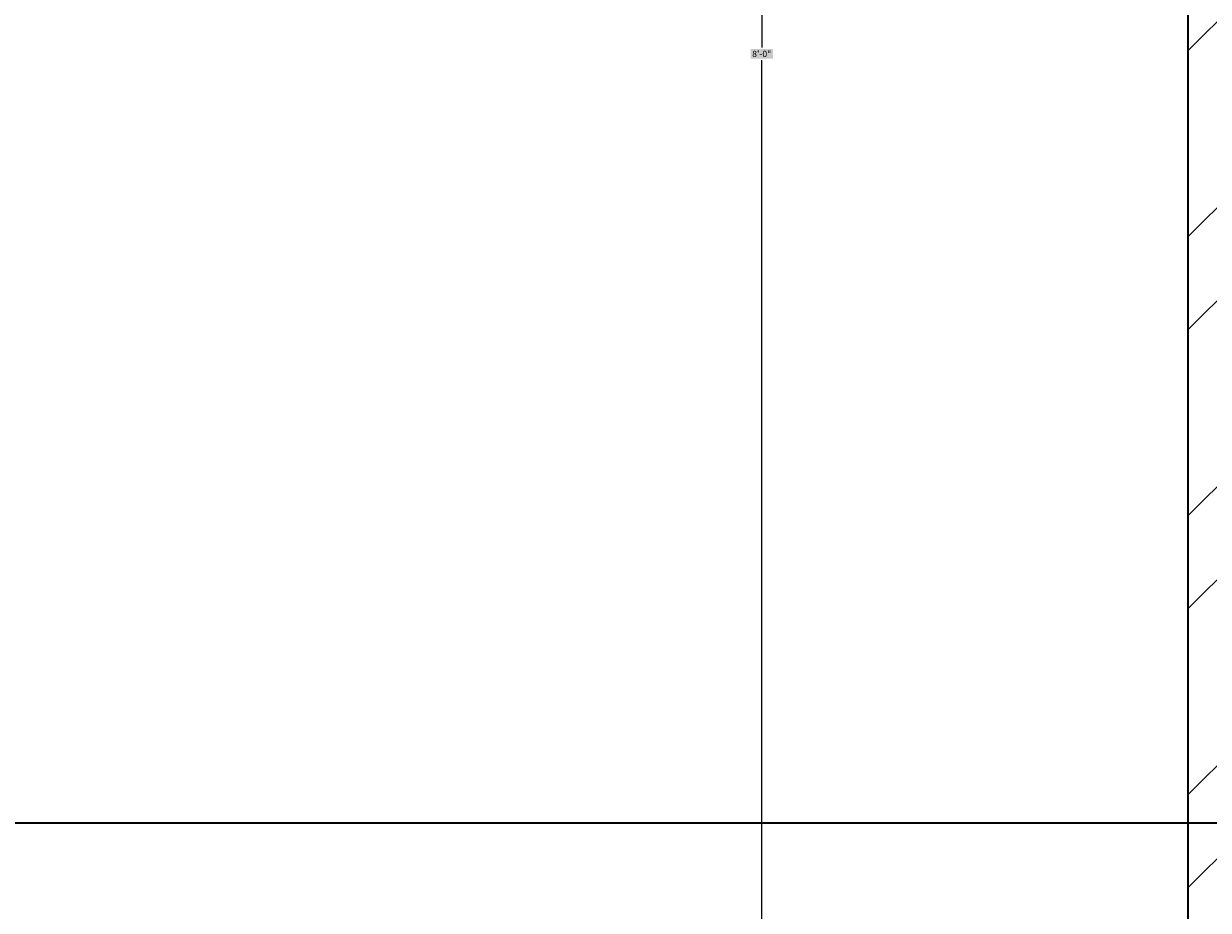
# Model space of a CAD drawing. Units: inches. Extents: x -301 to 715, y -607 to 364.
# Tile 34 of 141: x 101 to 135, y -466 to -441. Entities that reach past the tile are written whole.
import ezdxf

# ---------------------------------------------------------------- set-up
doc = ezdxf.new("R2010")
doc.units = ezdxf.units.IN
doc.header["$MEASUREMENT"] = 0
for name, color, linetype, lineweight in [('A-ANNO-DIMS', 2, 'Continuous', 18), ('A-SECT', 1, 'Continuous', 35), ('A-SECT-PATT', 8, 'Continuous', 13)]:
    doc.layers.add(name, color=color, linetype=linetype, lineweight=lineweight)
doc.styles.get("Standard").update_dxf_attribs({"font": 'arial.ttf'})
doc.dimstyles.get("Standard").update_dxf_attribs({"dimtxt": 0.18, "dimasz": 0.18, "dimexe": 0.18, "dimexo": 0.0625, "dimgap": 0.09, "dimtad": 0, "dimtih": 1, "dimtoh": 1, "dimdec": 1, "dimzin": 0, "dimdsep": 46, "dimlunit": 4, "dimtxsty": 'Standard', "dimcen": 0.09, "dimclrd": 3, "dimclre": 4, "dimclrt": 6, "dimadec": 0, "dimazin": 0, "dimtfac": 1, "dimtdec": 1, "dimtofl": 0, "dimtmove": 0, "dimatfit": 3, "dimfxl": 1, "dimtfill": 2, "dimtfillclr": 51, "dimtolj": 1, "dimtzin": 0, "dimarcsym": 0})
pattern_1 = [(45, (10.321, 33.8764), (-3.977476, 3.977476), []), (45, (12.973, 33.8764), (-3.977476, 3.977476), [])]

# ---------------------------------------------------------------- blocks, each defined once
blk = doc.blocks.new('*D176')
at = {"layer": 'A-ANNO-DIMS', "color": 4, "lineweight": -2, "transparency": 16777216}
for p, q in [((148.28, -324.477), (215.605, -324.477)), ((-15.22, -540.477), (215.605, -540.477))]:
    blk.add_line(p, q, dxfattribs=at)
at = {"layer": 'A-ANNO-DIMS', "color": 3, "lineweight": -2, "transparency": 16777216}
for p, q in [((215.425, -324.657), (215.425, -432.296)), ((215.425, -540.297), (215.425, -432.659))]:
    blk.add_line(p, q, dxfattribs=at)
at = {"layer": 'A-ANNO-DIMS', "color": 3, "transparency": 16777216}
for points in [[(215.395, -324.657), (215.455, -324.657), (215.425, -324.477)], [(215.395, -540.297), (215.455, -540.297), (215.425, -540.477)]]:
    blk.add_solid(points, dxfattribs=at)
at = {"layer": 'Defpoints', "color": 0, "transparency": 16777216}
for p in [(148.218, -324.477), (-15.282, -540.477), (215.425, -540.477)]:
    blk.add_point(p, dxfattribs=at)
at = {"layer": 'A-ANNO-DIMS', "color": 6, "transparency": 16777216, "insert": (215.425, -432.477), "char_height": 0.18, "attachment_point": 5, "bg_fill": 1, "box_fill_scale": 1.25, "bg_fill_color": 51, "bg_fill_transparency": 0}
blk.add_mtext('\\A1;18\'-0"', dxfattribs=at)
blk = doc.blocks.new('*D200')
at = {"layer": 'A-ANNO-DIMS', "color": 4, "lineweight": -2, "transparency": 16777216}
for p, q in [((412.955, -393.552), (121.926, -393.552)), ((412.955, -489.552), (121.926, -489.552))]:
    blk.add_line(p, q, dxfattribs=at)
at = {"layer": 'A-ANNO-DIMS', "color": 3, "lineweight": -2, "transparency": 16777216}
for p, q in [((122.106, -393.732), (122.106, -441.371)), ((122.106, -489.372), (122.106, -441.734))]:
    blk.add_line(p, q, dxfattribs=at)
at = {"layer": 'A-ANNO-DIMS', "color": 3, "transparency": 16777216}
for points in [[(122.076, -393.732), (122.136, -393.732), (122.106, -393.552)], [(122.076, -489.372), (122.136, -489.372), (122.106, -489.552)]]:
    blk.add_solid(points, dxfattribs=at)
at = {"layer": 'Defpoints', "color": 0, "transparency": 16777216}
for p in [(122.106, -393.552), (413.018, -393.552), (413.018, -489.552)]:
    blk.add_point(p, dxfattribs=at)
at = {"layer": 'A-ANNO-DIMS', "color": 6, "transparency": 16777216, "insert": (122.106, -441.552), "char_height": 0.18, "attachment_point": 5, "bg_fill": 1, "box_fill_scale": 1.25, "bg_fill_color": 51, "bg_fill_transparency": 0}
blk.add_mtext('\\A1;8\'-0"', dxfattribs=at)

msp = doc.modelspace()

# ---------------------------------------------------------------- hatches: boundary and pattern name
at = {"layer": 'A-SECT-PATT'}
h = msp.add_hatch(dxfattribs=at)
h.set_pattern_fill('ANSI32', color=256, scale=15)
h.set_pattern_definition(pattern_1)
h.paths.add_polyline_path([(-185.282, -324.477), (-199.282, -324.477), (-199.282, -329.477), (-194.282, -329.477), (-194.282, -353.477), (-185.282, -353.477)])
h.paths.add_polyline_path([(-185.282, -361.477), (-193.904, -361.477), (-193.982, -377.537), (-185.282, -377.537)])
h.paths.add_polyline_path([(143.218, -329.477), (148.218, -329.477), (148.218, -324.477), (134.255, -324.477), (134.255, -353.477), (143.218, -353.477)])
h.paths.add_polyline_path([(143.218, -361.477), (134.255, -361.477), (134.255, -377.477), (143.218, -377.477)])
h.paths.add_polyline_path([(-185.282, -439.477), (-194.282, -439.477), (-194.282, -463.477), (-185.282, -463.477)])
h.paths.add_polyline_path([(-185.282, -471.477), (-194.282, -471.477), (-194.282, -481.477), (-185.282, -481.477)])
h.paths.add_polyline_path([(-185.282, -463.477), (-194.282, -463.477), (-194.282, -466.477), (-185.282, -466.477)])
h.paths.add_polyline_path([(-185.282, -466.477), (-194.282, -466.477), (-194.282, -471.477), (-185.282, -471.477)])
h.paths.add_polyline_path([(-180.282, -481.477), (-185.282, -481.477), (-194.282, -481.477), (-199.282, -481.477), (-199.282, -493.477), (-180.282, -493.477)])
h.paths.add_polyline_path([(-175.282, -493.477), (-180.282, -493.477), (-199.282, -493.477), (-204.282, -493.477), (-204.282, -511.477), (-175.282, -511.477)])
h.paths.add_polyline_path([(-170.282, -511.477), (-175.282, -511.477), (-204.282, -511.477), (-209.282, -511.477), (-209.282, -535.477), (-170.282, -535.477)])
h.paths.add_polyline_path([(-35.282, -463.477), (-41.282, -463.477), (-41.282, -466.477), (-35.282, -466.477)])
h.paths.add_polyline_path([(-35.282, -466.477), (-41.282, -466.477), (-41.282, -471.477), (-35.282, -471.477)])
h.paths.add_polyline_path([(-35.282, -471.477), (-41.282, -471.477), (-41.282, -481.477), (-35.282, -481.477)])
h.paths.add_polyline_path([(-30.282, -481.477), (-46.282, -481.477), (-46.282, -493.477), (-30.282, -493.477)])
h.paths.add_polyline_path([(-25.282, -493.477), (-30.282, -493.477), (-46.282, -493.477), (-51.282, -493.477), (-51.282, -511.477), (-25.282, -511.477)])
h.paths.add_polyline_path([(-20.282, -511.477), (-25.282, -511.477), (-51.282, -511.477), (-56.282, -511.477), (-56.282, -535.477), (-20.282, -535.477)])
h.paths.add_polyline_path([(143.218, -463.477), (134.255, -463.477), (134.255, -466.477), (143.218, -466.477)])
h.paths.add_polyline_path([(143.218, -466.477), (134.255, -466.477), (134.255, -471.477), (143.218, -471.477)])
h.paths.add_polyline_path([(143.218, -471.477), (134.255, -471.477), (134.255, -481.477), (143.218, -481.477)])
h.paths.add_polyline_path([(148.255, -481.477), (143.255, -481.477), (134.255, -481.477), (129.255, -481.477), (129.255, -493.477), (148.255, -493.477)])
h.paths.add_polyline_path([(153.255, -493.477), (148.255, -493.477), (129.255, -493.477), (124.255, -493.477), (124.255, -511.477), (153.255, -511.477)])
h.paths.add_polyline_path([(158.255, -511.477), (153.255, -511.477), (124.255, -511.477), (119.255, -511.477), (119.255, -535.477), (158.255, -535.477)])
h = msp.add_hatch(dxfattribs=at)
h.set_pattern_fill('ANSI32', color=256, scale=15)
h.set_pattern_definition(pattern_1)
h.paths.add_polyline_path([(-35.282, -361.477), (-41.282, -361.477), (-41.282, -376.452), (-35.282, -376.452)])
h.paths.add_polyline_path([(143.218, -439.477), (134.255, -439.477), (134.255, -463.477), (143.218, -463.477)])

# ---------------------------------------------------------------- linework, layer by layer
at = {"layer": 'A-SECT'}
for p, q in [((134.255, -361.477), (134.255, -481.477)), ((-199.282, -463.477), (148.255, -463.477))]:
    msp.add_line(p, q, dxfattribs=at)

# ---------------------------------------------------------------- dimensions: what is measured, and where the dimension line sits
at = {"layer": 'A-ANNO-DIMS'}
for base, p1, p2, picture, middle in [((215.425, -540.477), (148.218, -324.477), (-15.282, -540.477), '*D176', (215.425, -432.477)), ((122.106, -393.552), (413.018, -489.552), (413.018, -393.552), '*D200', (122.106, -441.552))]:
    dim = msp.add_linear_dim(base=base, p1=p1, p2=p2, angle=90, dimstyle='Standard', override={"dimdec": 1, "dimlfac": 1, "dimrnd": 0, "dimzin": 1, "dimdsep": 46, "dimlunit": 4, "dimfrac": 2}, dxfattribs=at)
    dim.commit()
    dim.dimension.update_dxf_attribs({"geometry": picture, "text_midpoint": middle})

doc.saveas('drawing.dxf')
